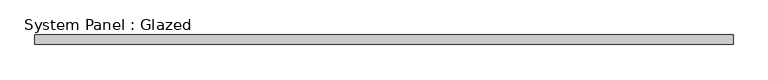
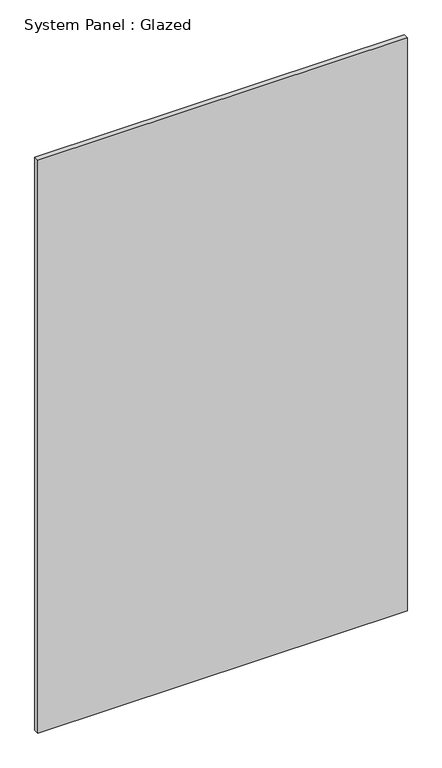
"""IFC4 building model written with IfcOpenShell, lengths in millimetres: plate geometry, System Panel : Glazed."""

from ifc_helpers import new_model, si_unit, origin, origin_with_axes, place, context, project, spatial, polyline, outline, extrude, source, transform, mapped, element, save


def system_panel_glazed_7a21471d(model_context):
    return source(origin(), model_context, "Body", "SweptSolid", [
        extrude(outline(polyline([(915.797, 24.5), (-915.797, 24.5), (-915.797, 49.5), (915.797, 49.5), (915.797, 24.5)])), origin_with_axes(), (0.0, 0.0, 1.0), 3000.0),
    ])


if __name__ == "__main__":
    model = new_model("IFC4")
    model_context = context("Model", 3, world=origin())
    ifc_project = project(units=[si_unit("LENGTHUNIT", "METRE", prefix="MILLI")], contexts=[model_context])
    site = spatial("IfcSite", under=ifc_project)
    building = spatial("IfcBuilding", under=site)
    placement = place(None, origin())
    system_panel_glazed_shape = system_panel_glazed_7a21471d(model_context)
    element("IfcPlate", 1, ObjectType="System Panel : Glazed", at=placement, inside=building, context=model_context, shape_type="MappedRepresentation", body=[
        mapped(system_panel_glazed_shape, transform((0.0, 0.0, 0.0), x_axis=(1.0, 0.0, 0.0), y_axis=(0.0, 1.0, 0.0), z_axis=(0.0, 0.0, 1.0))),
    ])
    save(model, "model.ifc")

# Revit data of these elements
# Type "System Panel : Glazed"
#   Keynote = "H11"
#   Construction Type Id = "GSP4R"
#   Analytic Construction = "1/8 in Pilkington single glazing"
#   Visual Light Transmittance = 0.9
#   Solar Heat Gain Coefficient = 0.86
#   Heat Transfer Coefficient (U) = 6.7069 W/(m²·K)
#   Define Thermal Properties by = 1
# Element 1 (IfcPlate, "System Panel : Glazed")
#   Materials on its faces: "Glass"
# Materials
#   "Glass": class "Glass", colour RGB 0 128 192, transparency 0.9, Description = "Soda Lime Glass", Cost = 0
